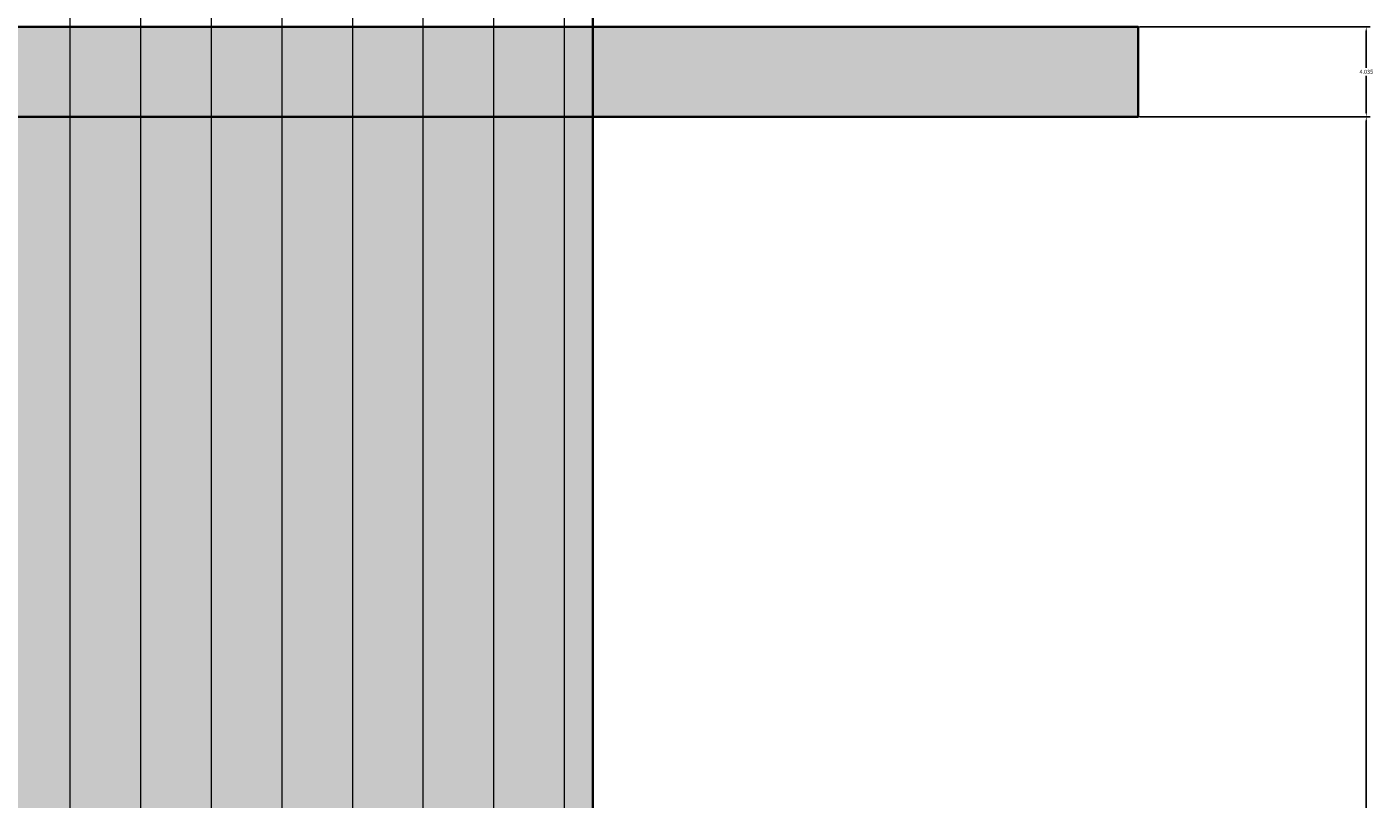
# Model space of a CAD drawing. Units: millimetres. Extents: x 446512 to 447461, y 70395 to 70610.
# Tile 38 of 39: x 447401 to 447461, y 70472 to 70507. Entities that reach past the tile are written whole.
import ezdxf

# ---------------------------------------------------------------- set-up
doc = ezdxf.new("R2010")
doc.units = ezdxf.units.MM
for name, color, linetype, lineweight in [('A-ANNO-DIMS', 2, 'Continuous', 18), ('A-FURN', 7, 'Continuous', 35), ('A-FURN-PATT', 38, 'Continuous', 13)]:
    doc.layers.add(name, color=color, linetype=linetype, lineweight=lineweight)
doc.styles.get("Standard").update_dxf_attribs({"font": 'arial.ttf'})
doc.dimstyles.get("Standard").update_dxf_attribs({"dimtxt": 0.18, "dimasz": 0.18, "dimexe": 0.18, "dimexo": 0.0625, "dimgap": 0.09, "dimtad": 0, "dimtih": 1, "dimtoh": 1, "dimdec": 4, "dimzin": 0, "dimdsep": 46, "dimtxsty": 'Standard', "dimcen": 0.09, "dimadec": 0, "dimazin": 0, "dimtfac": 1, "dimtdec": 4, "dimtofl": 0, "dimtmove": 0, "dimatfit": 3, "dimfxl": 1, "dimtolj": 1, "dimtzin": 0, "dimarcsym": 0})

# ---------------------------------------------------------------- blocks, each defined once
blk = doc.blocks.new('*D69')
at = {"layer": 'A-ANNO-DIMS', "color": 0, "lineweight": -2, "transparency": 16777216}
for p, q in [((447450.594, 70502.515), (447460.962, 70502.515)), ((447460.782, 70502.335), (447460.782, 70469.583)), ((447460.782, 70436.468), (447460.782, 70469.219)), ((447450.594, 70436.288), (447460.962, 70436.288))]:
    blk.add_line(p, q, dxfattribs=at)
at = {"layer": 'A-ANNO-DIMS', "color": 0, "transparency": 16777216}
for points in [[(447460.752, 70502.335), (447460.812, 70502.335), (447460.782, 70502.515)], [(447460.752, 70436.468), (447460.812, 70436.468), (447460.782, 70436.288)]]:
    blk.add_solid(points, dxfattribs=at)
at = {"layer": 'Defpoints', "color": 0, "transparency": 16777216}
for p in [(447450.532, 70502.515), (447460.782, 70502.515), (447450.532, 70436.288)]:
    blk.add_point(p, dxfattribs=at)
at = {"layer": 'A-ANNO-DIMS', "color": 0, "transparency": 16777216, "insert": (447460.782, 70469.401), "char_height": 0.18, "attachment_point": 5}
blk.add_mtext('\\A1;66.23', dxfattribs=at)
blk = doc.blocks.new('*D70')
at = {"layer": 'A-ANNO-DIMS', "color": 0, "lineweight": -2, "transparency": 16777216}
for p, q in [((447450.594, 70506.55), (447460.962, 70506.55)), ((447460.782, 70506.37), (447460.782, 70504.714)), ((447460.782, 70502.695), (447460.782, 70504.35)), ((447450.594, 70502.515), (447460.962, 70502.515))]:
    blk.add_line(p, q, dxfattribs=at)
at = {"layer": 'A-ANNO-DIMS', "color": 0, "transparency": 16777216}
for points in [[(447460.752, 70506.37), (447460.812, 70506.37), (447460.782, 70506.55)], [(447460.752, 70502.695), (447460.812, 70502.695), (447460.782, 70502.515)]]:
    blk.add_solid(points, dxfattribs=at)
at = {"layer": 'Defpoints', "color": 0, "transparency": 16777216}
for p in [(447450.532, 70506.55), (447460.782, 70506.55), (447450.532, 70502.515)]:
    blk.add_point(p, dxfattribs=at)
at = {"layer": 'A-ANNO-DIMS', "color": 0, "transparency": 16777216, "insert": (447460.782, 70504.532), "char_height": 0.18, "attachment_point": 5}
blk.add_mtext('\\A1;4.035', dxfattribs=at)

msp = doc.modelspace()

# ---------------------------------------------------------------- hatches: boundary and pattern name
at = {"layer": 'A-FURN-PATT'}
h = msp.add_hatch(dxfattribs=at)
h.set_pattern_fill('ANSI31', color=256, angle=45)
h.set_pattern_definition([(90, (127.5626, 0), (-3.175, 0), [])])
h.paths.add_polyline_path([(447426.0142, 70599.7147), (447365.4251, 70599.7147), (447365.4251, 70405.3145), (447426.0142, 70405.3145)])
h = msp.add_hatch(color=256, dxfattribs=at)
h.dxf.hatch_style = 1
h.paths.add_polyline_path([(447365.4251, 70506.5496), (447340.0494, 70506.5496), (447340.0494, 70502.5146), (447365.4251, 70502.5146)])
h.paths.add_polyline_path([(447450.5318, 70506.5496), (447426.0142, 70506.5496), (447426.0142, 70502.5146), (447450.5318, 70502.5146)])
h.paths.add_polyline_path([(447426.0142, 70506.5496), (447365.4251, 70506.5496), (447365.4251, 70502.5146), (447426.0142, 70502.5146)])
h = msp.add_hatch(color=256, dxfattribs=at)
h.dxf.hatch_style = 1
h.paths.add_polyline_path([(447426.0142, 70502.5146), (447365.4251, 70502.5146), (447365.4251, 70436.2876), (447426.0142, 70436.2876)])

# ---------------------------------------------------------------- linework, layer by layer
at = {"layer": 'A-FURN'}
msp.add_line((447426.0142, 70405.3145), (447426.0142, 70599.7147), dxfattribs=at)
msp.add_lwpolyline([(447340.0494, 70506.5496), (447450.5318, 70506.5496), (447450.5318, 70502.5146), (447340.0494, 70502.5146)], close=True, dxfattribs=at)

# ---------------------------------------------------------------- dimensions: what is measured, and where the dimension line sits
at = {"layer": 'A-ANNO-DIMS'}
for base, p1, p2, override, picture, middle in [((447460.7818, 70506.5496), (447450.5318, 70502.5146), (447450.5318, 70506.5496), {"dimdec": 3, "dimlfac": 1, "dimrnd": 0, "dimzin": 0, "dimdsep": 46, "dimlunit": 2}, '*D70', (447460.7818, 70504.5321)), ((447460.7818, 70502.5146), (447450.5318, 70436.2876), (447450.5318, 70502.5146), {"dimdec": 2, "dimlfac": 1, "dimrnd": 0, "dimzin": 0, "dimdsep": 46, "dimlunit": 2}, '*D69', (447460.7818, 70469.4011))]:
    dim = msp.add_linear_dim(base=base, p1=p1, p2=p2, angle=90, dimstyle='Standard', override=override, dxfattribs=at)
    dim.commit()
    dim.dimension.update_dxf_attribs({"geometry": picture, "text_midpoint": middle})

doc.saveas('drawing.dxf')
